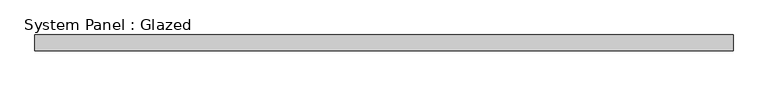
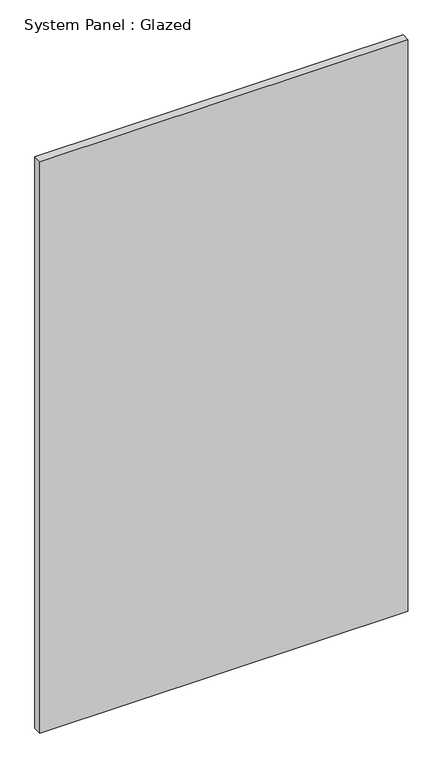
"""IFC4 building model written with IfcOpenShell, lengths in millimetres: plate geometry, System Panel : Glazed."""

from ifc_helpers import new_model, si_unit, origin, origin_with_axes, place, context, project, spatial, polyline, outline, extrude, source, transform, mapped, element, save


def system_panel_glazed_8012c4e8(model_context):
    return source(origin(), model_context, "Body", "SweptSolid", [
        extrude(outline(polyline([(561.975, 19.05), (-561.975, 19.05), (-561.975, 44.45), (561.975, 44.45), (561.975, 19.05)])), origin_with_axes(), (0.0, 0.0, 1.0), 1843.7905078),
    ])


if __name__ == "__main__":
    model = new_model("IFC4")
    model_context = context("Model", 3, world=origin())
    ifc_project = project(units=[si_unit("LENGTHUNIT", "METRE", prefix="MILLI")], contexts=[model_context])
    site = spatial("IfcSite", under=ifc_project)
    building = spatial("IfcBuilding", under=site)
    placement = place(None, origin())
    system_panel_glazed_shape = system_panel_glazed_8012c4e8(model_context)
    element("IfcPlate", 1, ObjectType="System Panel : Glazed", at=placement, inside=building, context=model_context, shape_type="MappedRepresentation", body=[
        mapped(system_panel_glazed_shape, transform((0.0, 0.0, 0.0), x_axis=(1.0, 0.0, 0.0), y_axis=(0.0, 1.0, 0.0), z_axis=(0.0, 0.0, 1.0))),
    ])
    save(model, "model.ifc")

# Revit data of these elements
# Type "System Panel : Glazed"
#   Construction Type Id = "GSP4R"
#   Analytic Construction = "1/8 in Pilkington single glazing"
#   Visual Light Transmittance = 0.9
#   Solar Heat Gain Coefficient = 0.86
#   Heat Transfer Coefficient (U) = 1.18115 BTU/(h·ft²·°F)
#   Define Thermal Properties by = 1
# Element 1 (IfcPlate, "System Panel : Glazed")
#   Materials on its faces: "Glass"
# Materials
#   "Glass": class "Glass", colour RGB 0 128 192, transparency 0.75, Description = "Soda Lime Glass", Cost = 0
